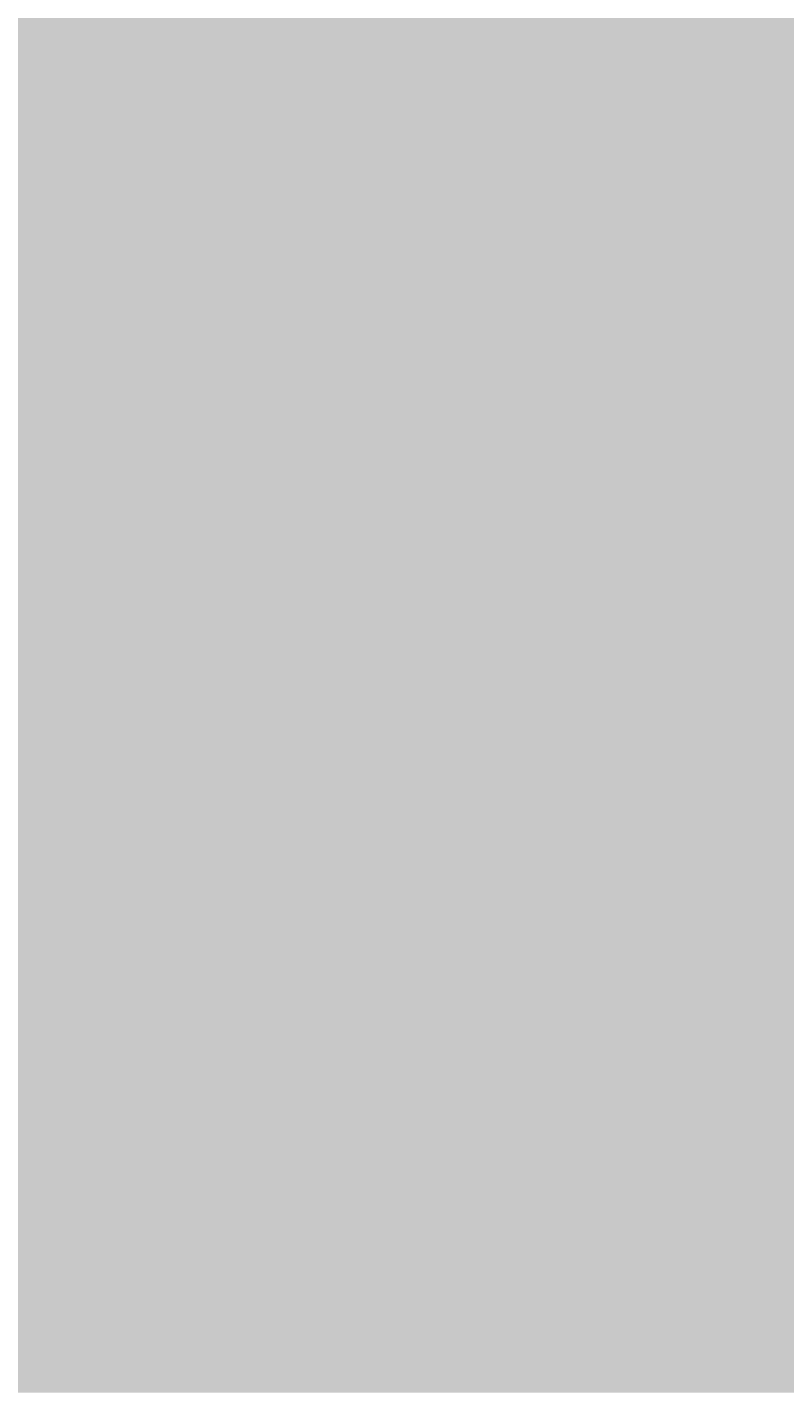
# Model space of a CAD drawing. Units: inches. Extents: x 84 to 1044, y -280 to 906.
# Tile 86 of 105: x 856 to 870, y 400 to 426. Entities that reach past the tile are written whole.
import ezdxf

# ---------------------------------------------------------------- set-up
doc = ezdxf.new("R2010")
doc.units = ezdxf.units.IN
doc.layers.add('A-ANNO-DIMS', color=2, linetype='Continuous', lineweight=18)
doc.layers.add('L-PLNT-PATT', color=9, linetype='Continuous', lineweight=9, true_color=0xafd9aa)
doc.styles.get("Standard").update_dxf_attribs({"font": 'arial.ttf'})
doc.dimstyles.get("Standard").update_dxf_attribs({"dimtxt": 0.18, "dimasz": 0.18, "dimexe": 0.18, "dimexo": 0.0625, "dimgap": 0.09, "dimtad": 0, "dimtih": 1, "dimtoh": 1, "dimdec": 4, "dimzin": 0, "dimdsep": 46, "dimtxsty": 'Standard', "dimcen": 0.09, "dimadec": 0, "dimazin": 0, "dimtfac": 1, "dimtdec": 4, "dimtofl": 0, "dimtmove": 0, "dimatfit": 3, "dimfxl": 1, "dimtolj": 1, "dimtzin": 0, "dimarcsym": 0})

# ---------------------------------------------------------------- blocks, each defined once
blk = doc.blocks.new('*D62')
at = {"layer": 'A-ANNO-DIMS', "color": 0, "lineweight": -2, "transparency": 16777216}
for p, q in [((203.179, 709.183), (203.179, 905.9)), ((203.359, 905.72), (549.232, 905.72)), ((895.894, 905.72), (550.021, 905.72)), ((896.074, 400.183), (896.074, 905.9))]:
    blk.add_line(p, q, dxfattribs=at)
at = {"layer": 'A-ANNO-DIMS', "color": 0, "transparency": 16777216}
for points in [[(203.359, 905.75), (203.359, 905.69), (203.179, 905.72)], [(895.894, 905.75), (895.894, 905.69), (896.074, 905.72)]]:
    blk.add_solid(points, dxfattribs=at)
at = {"layer": 'Defpoints', "color": 0, "transparency": 16777216}
for p in [(896.074, 905.72), (203.179, 709.12), (896.074, 400.12)]:
    blk.add_point(p, dxfattribs=at)
at = {"layer": 'A-ANNO-DIMS', "color": 0, "transparency": 16777216, "insert": (549.627, 905.72), "char_height": 0.18, "attachment_point": 5}
blk.add_mtext('\\A1;692.9', dxfattribs=at)
blk = doc.blocks.new('*D63')
at = {"layer": 'A-ANNO-DIMS', "color": 0, "lineweight": -2, "transparency": 16777216}
for p, q in [((833.136, 709.12), (1043.768, 709.12)), ((1043.588, 708.94), (1043.588, 400.302)), ((1043.588, 91.3), (1043.588, 399.938)), ((896.136, 91.12), (1043.768, 91.12))]:
    blk.add_line(p, q, dxfattribs=at)
at = {"layer": 'A-ANNO-DIMS', "color": 0, "transparency": 16777216}
for points in [[(1043.558, 708.94), (1043.618, 708.94), (1043.588, 709.12)], [(1043.558, 91.3), (1043.618, 91.3), (1043.588, 91.12)]]:
    blk.add_solid(points, dxfattribs=at)
at = {"layer": 'Defpoints', "color": 0, "transparency": 16777216}
for p in [(833.074, 709.12), (1043.588, 709.12), (896.074, 91.12)]:
    blk.add_point(p, dxfattribs=at)
at = {"layer": 'A-ANNO-DIMS', "color": 0, "transparency": 16777216, "insert": (1043.588, 400.12), "char_height": 0.18, "attachment_point": 5}
blk.add_mtext('\\A1;618', dxfattribs=at)

msp = doc.modelspace()

# ---------------------------------------------------------------- hatches: boundary and pattern name
at = {"layer": 'L-PLNT-PATT', "transparency": 33554597}
h = msp.add_hatch(color=256, dxfattribs=at)
h.dxf.hatch_style = 1
h.paths.add_polyline_path([(896.074, 511.12), (704.074, 511.12), (704.074, 491.62), (704.074, 419.62), (704.074, 400.12), (833.074, 400.12), (896.074, 400.12)])

# ---------------------------------------------------------------- dimensions: what is measured, and where the dimension line sits
at = {"layer": 'A-ANNO-DIMS'}
dim = msp.add_linear_dim(base=(896.074, 905.72), p1=(203.179, 709.12), p2=(896.074, 400.12), dimstyle='Standard', override={"dimdec": 1, "dimlfac": 1, "dimrnd": 0, "dimzin": 0, "dimdsep": 46, "dimlunit": 2}, dxfattribs=at)
dim.commit()
dim.dimension.update_dxf_attribs({"geometry": '*D62', "text_midpoint": (549.627, 905.72)})
dim = msp.add_linear_dim(base=(1043.588, 709.12), p1=(896.074, 91.12), p2=(833.074, 709.12), angle=90, dimstyle='Standard', override={"dimdec": 0, "dimlfac": 1, "dimrnd": 0, "dimzin": 0, "dimdsep": 46, "dimlunit": 2}, dxfattribs=at)
dim.commit()
dim.dimension.update_dxf_attribs({"geometry": '*D63', "text_midpoint": (1043.588, 400.12)})

doc.saveas('drawing.dxf')
